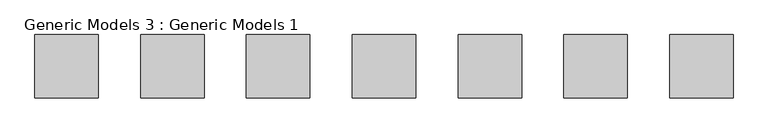
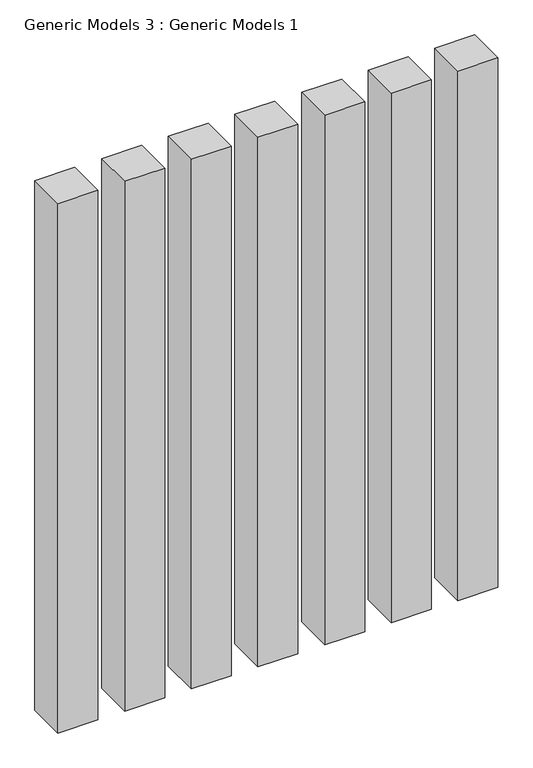
"""IFC4 building model written with IfcOpenShell, lengths in millimetres: proxy geometry, Generic Models 3 : Generic Models 1."""

from ifc_helpers import new_model, si_unit, origin, origin_with_axes, place, context, project, spatial, polyline, outline, extrude, source, transform, mapped, element, save


def generic_models_3_generic_models_1_029f251b(model_context):
    return source(origin(), model_context, "Body", "SweptSolid", [
        extrude(outline(polyline([(-9705.9453682, -2836.165108), (-9934.5453682, -2836.165108), (-9934.5453682, -2607.565108), (-9705.9453682, -2607.565108), (-9705.9453682, -2836.165108)])), origin_with_axes(), (0.0, 0.0, 1.0), 3200.4),
        extrude(outline(polyline([(-9324.9453682, -2836.165108), (-9553.5453682, -2836.165108), (-9553.5453682, -2607.565108), (-9324.9453682, -2607.565108), (-9324.9453682, -2836.165108)])), origin_with_axes(), (0.0, 0.0, 1.0), 3200.4),
        extrude(outline(polyline([(-8943.9453682, -2836.165108), (-9172.5453682, -2836.165108), (-9172.5453682, -2607.565108), (-8943.9453682, -2607.565108), (-8943.9453682, -2836.165108)])), origin_with_axes(), (0.0, 0.0, 1.0), 3200.4),
        extrude(outline(polyline([(-8562.9453682, -2836.165108), (-8791.5453682, -2836.165108), (-8791.5453682, -2607.565108), (-8562.9453682, -2607.565108), (-8562.9453682, -2836.165108)])), origin_with_axes(), (0.0, 0.0, 1.0), 3200.4),
        extrude(outline(polyline([(-8181.9453682, -2836.165108), (-8410.5453682, -2836.165108), (-8410.5453682, -2607.565108), (-8181.9453682, -2607.565108), (-8181.9453682, -2836.165108)])), origin_with_axes(), (0.0, 0.0, 1.0), 3200.4),
        extrude(outline(polyline([(-7800.9453682, -2836.165108), (-8029.5453682, -2836.165108), (-8029.5453682, -2607.565108), (-7800.9453682, -2607.565108), (-7800.9453682, -2836.165108)])), origin_with_axes(), (0.0, 0.0, 1.0), 3200.4),
        extrude(outline(polyline([(-7419.9453682, -2836.165108), (-7648.5453682, -2836.165108), (-7648.5453682, -2607.565108), (-7419.9453682, -2607.565108), (-7419.9453682, -2836.165108)])), origin_with_axes(), (0.0, 0.0, 1.0), 3200.4),
    ])


if __name__ == "__main__":
    model = new_model("IFC4")
    model_context = context("Model", 3, world=origin())
    ifc_project = project(units=[si_unit("LENGTHUNIT", "METRE", prefix="MILLI")], contexts=[model_context])
    site = spatial("IfcSite", under=ifc_project)
    building = spatial("IfcBuilding", under=site)
    placement = place(None, origin())
    generic_models_3_generic_models_1_shape = generic_models_3_generic_models_1_029f251b(model_context)
    element("IfcBuildingElementProxy", 1, Name="Generic Models 3 : Generic Models 1", ObjectType="Generic Models 3 : Generic Models 1", at=placement, inside=building, context=model_context, shape_type="MappedRepresentation", body=[
        mapped(generic_models_3_generic_models_1_shape, transform((0.0, 0.0, 0.0), x_axis=(1.0, 0.0, 0.0), y_axis=(0.0, 1.0, 0.0), z_axis=(0.0, 0.0, 1.0))),
    ])
    save(model, "model.ifc")

# Revit data of these elements
# Element 1 (IfcBuildingElementProxy, "Generic Models 3 : Generic Models 1")
#   Materials on its faces: "0 olive green"
# Materials
#   "0 olive green": class "Generic", colour RGB 120 120 120, transparency 0, Cost = 0
